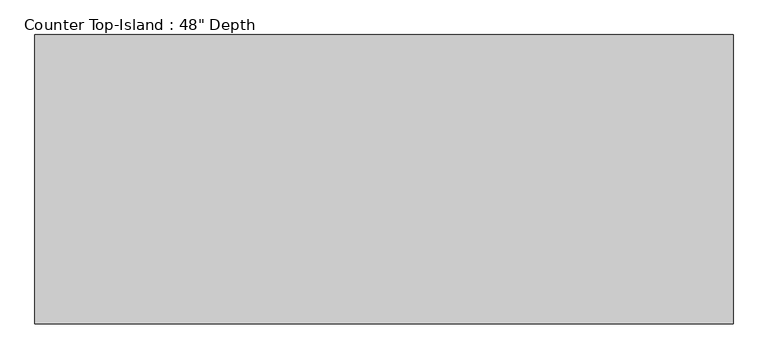
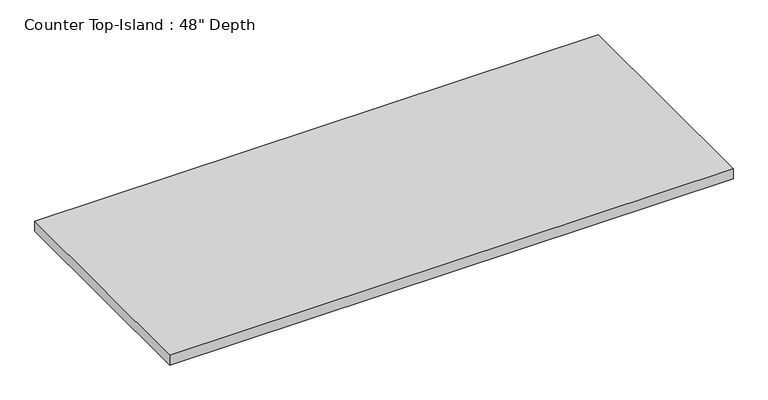
"""IFC4 building model written with IfcOpenShell, lengths in millimetres: furniture geometry."""

from ifc_helpers import new_model, si_unit, frame, origin, place, context, project, spatial, polyline, outline, extrude, source, transform, mapped, element, save


def furniture_0b3f2853(model_context):
    return source(origin(), model_context, "Body", "SweptSolid", [
        extrude(outline(polyline([(914.0764432, 25.4), (914.0764432, -851.5682571), (-1200.4622951, -851.5682571), (-1200.4622951, 25.4), (914.0764432, 25.4)])), frame((0.0, 0.0, 876.3), z_axis=(0.0, 0.0, 1.0), x_axis=(1.0, 0.0, 0.0)), (0.0, 0.0, 1.0), 38.1),
    ])


if __name__ == "__main__":
    model = new_model("IFC4")
    model_context = context("Model", 3, world=origin())
    ifc_project = project(units=[si_unit("LENGTHUNIT", "METRE", prefix="MILLI")], contexts=[model_context])
    site = spatial("IfcSite", under=ifc_project)
    building = spatial("IfcBuilding", under=site)
    placement = place(None, origin())
    furniture_shape = furniture_0b3f2853(model_context)
    element("IfcFurniture", 1, ObjectType="Counter Top-Island : 48\" Depth", at=placement, inside=building, context=model_context, shape_type="MappedRepresentation", body=[
        mapped(furniture_shape, transform((0.0, 0.0, 0.0), x_axis=(1.0, 0.0, 0.0), y_axis=(0.0, 1.0, 0.0), z_axis=(0.0, 0.0, 1.0))),
    ])
    save(model, "model.ifc")

# Revit data of these elements
# Type "Counter Top-Island : 48\" Depth"
#   Assembly Code = "C1030400"
#   Counter Thickness = 0' - 1 1/2"
#   Depth [instance default] = 4' - 2"
#   Height = 3' - 0"
#   Length [instance default] = 8' - 0"
#   Counter Top Material = none
#   Default Elevation = 0
# Element 1 (IfcFurniture, "Counter Top-Island : 48\" Depth")
#   Depth = 2' - 10.52631"
#   Length = 6' - 11.24956"
#   Materials on its faces: "Counter Top"
# Materials
#   "Counter Top": class "Wood", colour RGB 226 177 128, transparency 0
